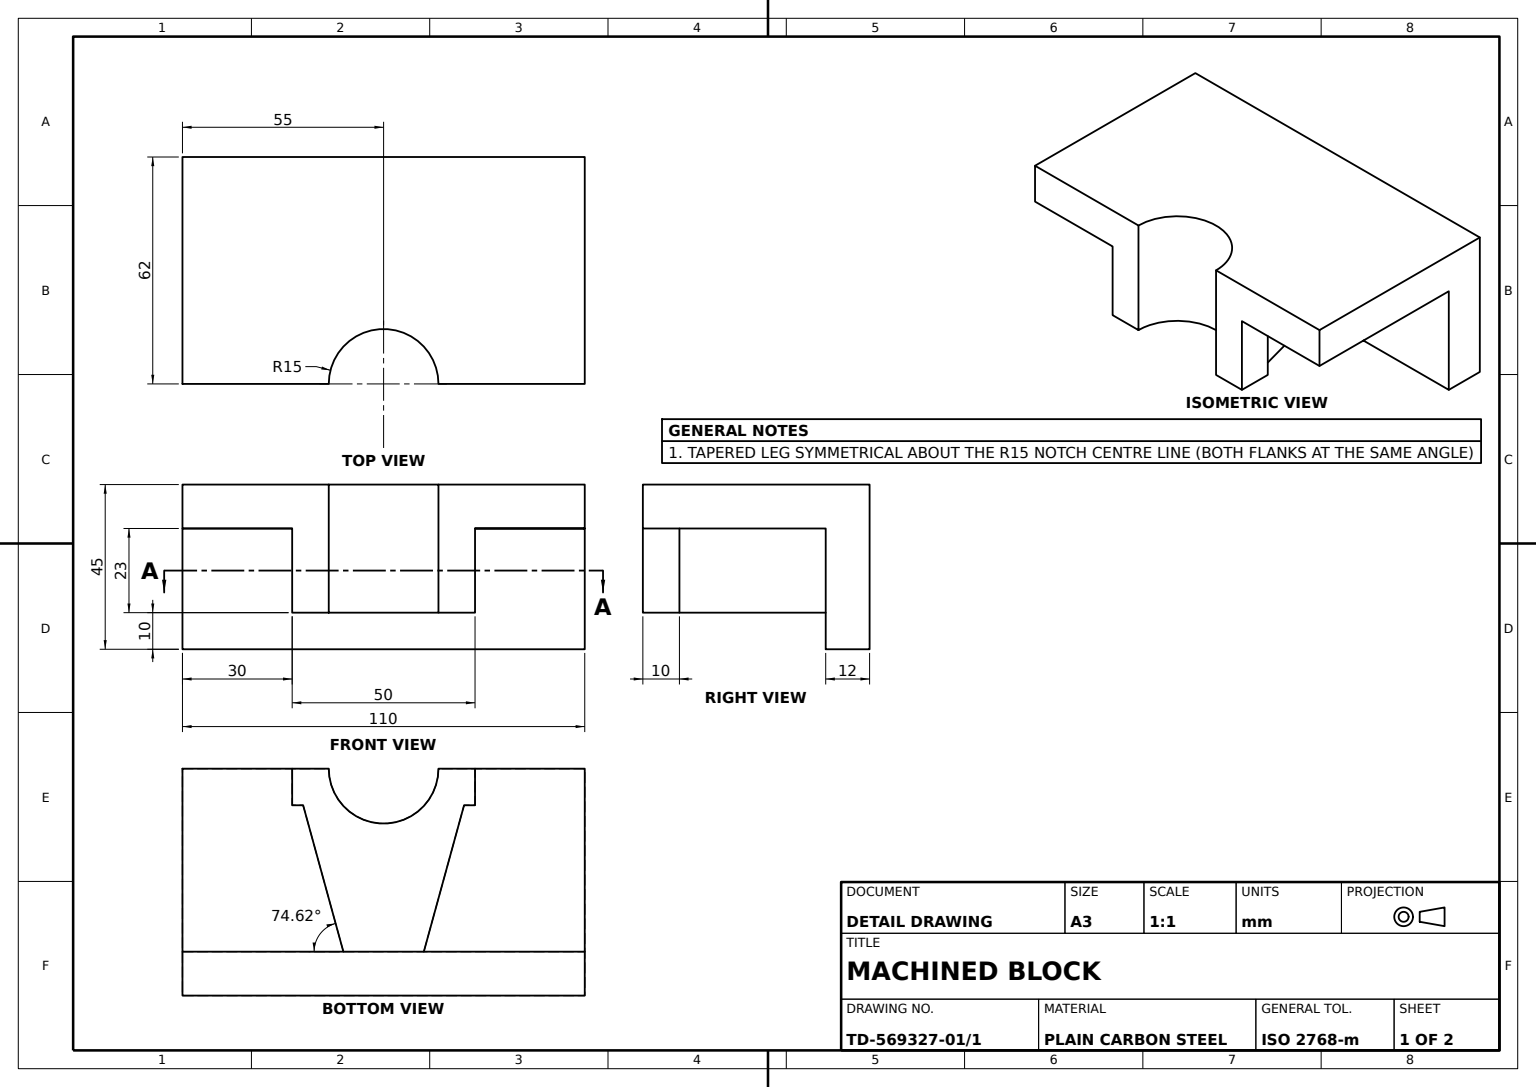
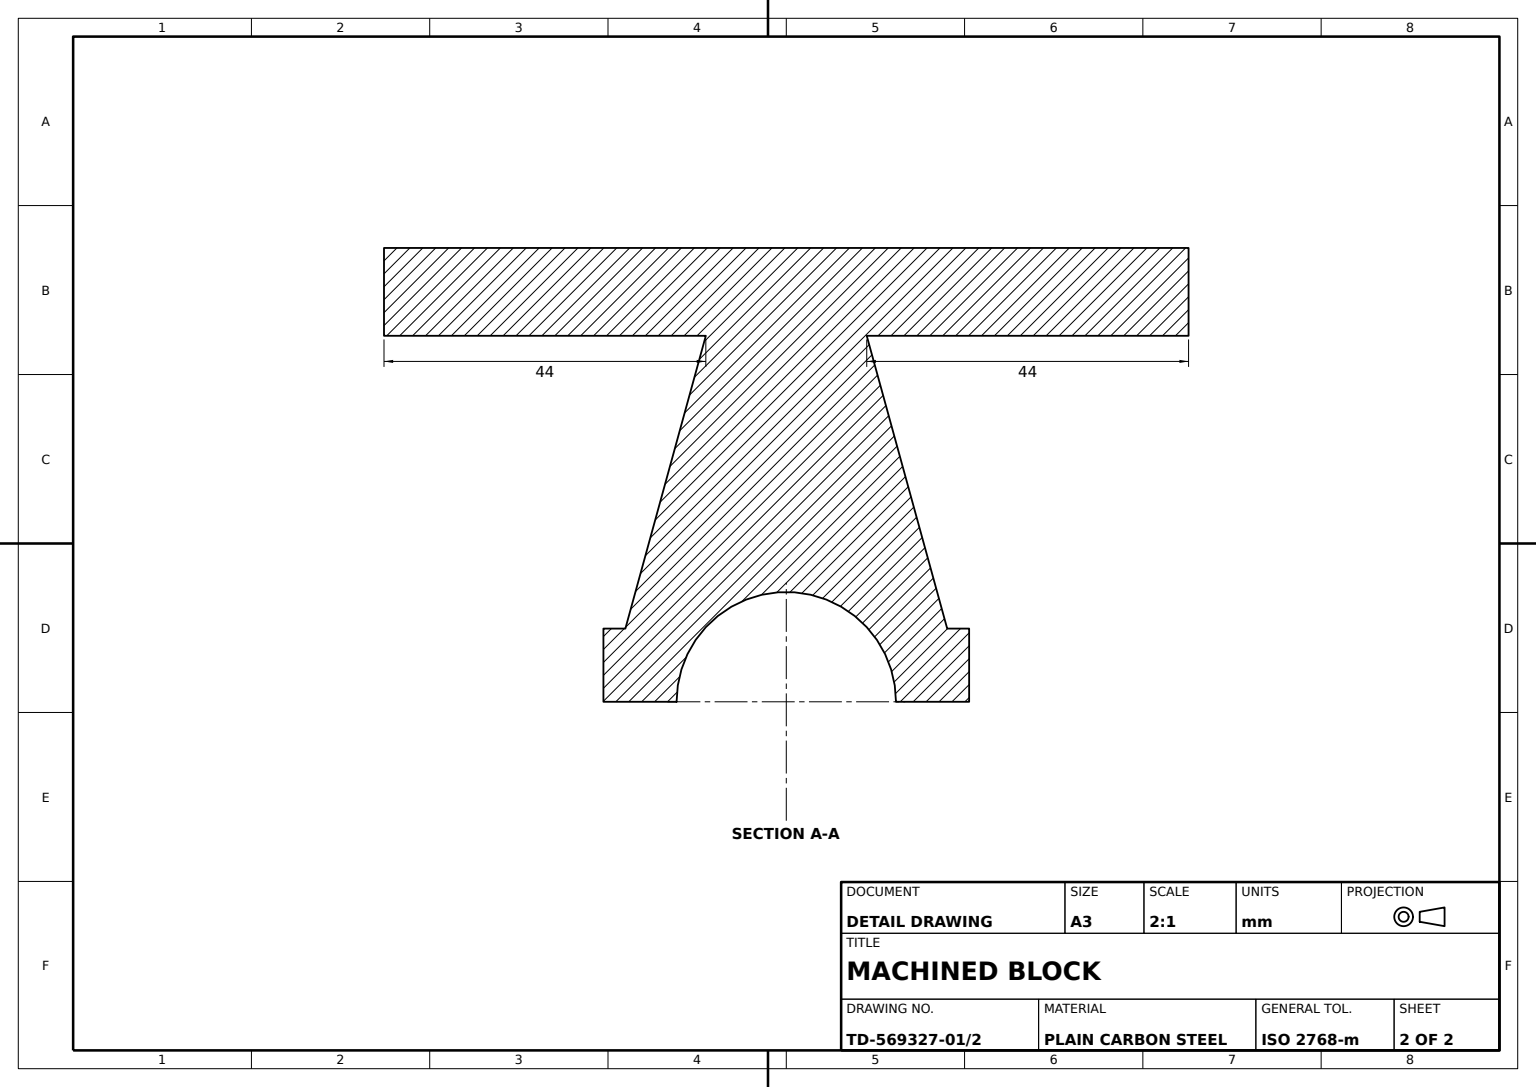
SolidWorks part; units mm, degrees
material "Plain Carbon Steel"
ref_plane "Front Plane" through (0, 0, 0) normal (0, 0, 1) x (1, 0, 0)
ref_plane "Top Plane" through (0, 0, 0) normal (0, 1, 0) x (1, 0, 0)
ref_plane "Right Plane" through (0, 0, 0) normal (1, 0, 0) x (0, 0, -1)
sketch "Base Plate Sketch" plane through (0, 0, 0) normal (0, 0, 1) x (1, 0, 0)
  line L0 (0, 0) -> (110, 0)
  line L1 (110, 0) -> (110, 45)
  line L2 (110, 45) -> (0, 45)
  line L3 (0, 45) -> (0, 0)
  dimension "D1" = 110
  dimension "D2" = 45
extrude "Base Plate" add sketch "Base Plate Sketch" along normal blind 12
sketch "Second Block Sketch" plane through (0, 45, 0) normal (0, 1, 0) x (1, 0, 0)
  line L0 (110, -12) -> (110, -62)
  line L1 (110, -62) -> (0, -62)
  line L2 (0, -62) -> (0, -12)
  line L3 (0, -12) -> (110, -12)
  line L5 (110, 0) -> (0, 0) construction
  dimension "D1" = 62
extrude "Second Block" add sketch "Second Block Sketch" against normal blind 12
sketch "Leg Profile Sketch" plane through (0, 33, 0) normal (0, -1, 0) x (1, 0, 0)
  line L1 (0, 62) -> (110, 62) construction
  line L3 (80, 62) -> (80, 52)
  line L5 (30, 52) -> (30, 62)
  line L6 (55, 12) -> (44, 12)
  line L7 (110, 12) -> (0, 12) construction
  line L8 (30, 62) -> (40, 62)
  line L9 (33, 52) -> (44, 12)
  line L10 (30, 52) -> (33, 52)
  line L11 (55, 12) -> (66, 12)
  line L12 (66, 12) -> (77, 52)
  line L13 (77, 52) -> (80, 52)
  line L14 (70, 62) -> (80, 62)
  line L15 (110, 62) -> (110, 12) construction
  arc A0 (40, 62) -> (70, 62) centre (55, 62) ccw
  dimension "D1" = 30
  dimension "D2" = 15
  dimension "D3" = 30
  dimension "D4" = 33
  dimension "D5" = 44
extrude "Leg Profile Boss" add sketch "Leg Profile Sketch" along normal blind 23
sketch "Semicircular Notch Sketch" plane through (0, 33, 0) normal (0, -1, 0) x (1, 0, 0)
  line L0 (40, 62) -> (70, 62)
  arc A0 (40, 62) -> (70, 62) centre (55, 62) ccw
  dimension "D1" = 30
extrude "Semicircular Notch Cut" cut sketch "Semicircular Notch Sketch" against normal blind 12
